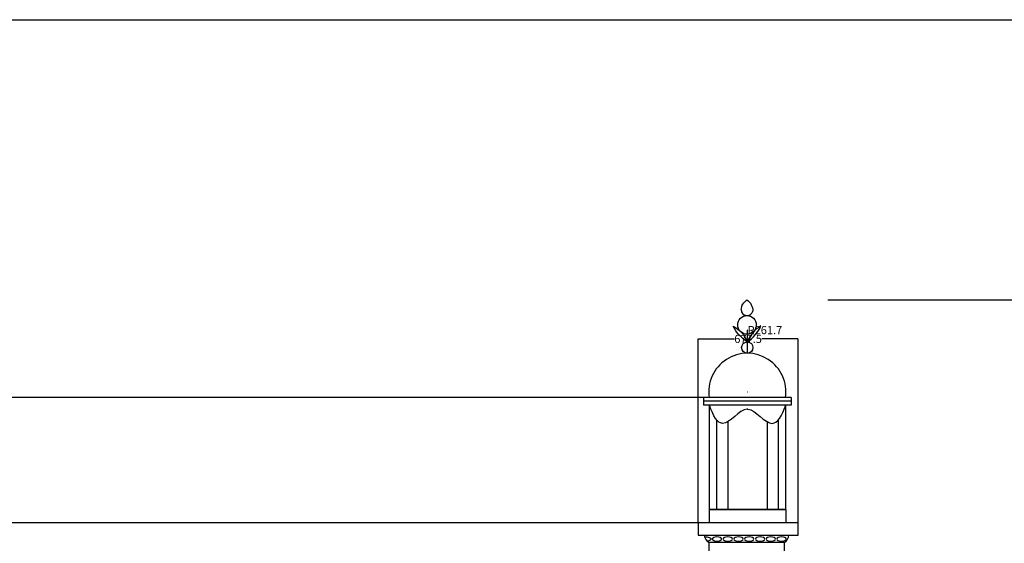
# Model space of a CAD drawing. Units: millimetres. Extents: x 8570 to 49085, y 3782 to 24863.
# Tile 11 of 15: x 28488 to 35169, y 17835 to 21387. Entities that reach past the tile are written whole.
import ezdxf

# ---------------------------------------------------------------- set-up
doc = ezdxf.new("R2010")
doc.units = ezdxf.units.MM
doc.header["$MEASUREMENT"] = 0
doc.header["$PDMODE"] = 3
doc.layers.add('A-ANNO-DIMS', color=2, linetype='Continuous', lineweight=18)
doc.layers.add('A-ELEV-MNRT', color=7, linetype='Continuous', lineweight=30)
doc.styles.get("Standard").update_dxf_attribs({"font": 'arial.ttf'})
doc.dimstyles.get("Standard").update_dxf_attribs({"dimtxt": 55, "dimasz": 0.18, "dimexe": 0.18, "dimexo": 0.0625, "dimgap": 0.09, "dimtad": 0, "dimtih": 1, "dimtoh": 1, "dimdec": 0, "dimzin": 0, "dimdsep": 46, "dimtxsty": 'Standard', "dimcen": 0.09, "dimadec": 0, "dimazin": 0, "dimtfac": 1, "dimtdec": 0, "dimtofl": 0, "dimtmove": 0, "dimatfit": 3, "dimfxl": 1, "dimtolj": 1, "dimtzin": 0, "dimarcsym": 0})

# ---------------------------------------------------------------- blocks, each defined once
blk = doc.blocks.new('MINARET-ELEV')
for p, q in [((851, 12922), (257.5, 12922)), ((257.5, 12922), (257.5, 12872)), ((851, 12897), (257.5, 12897)), ((851, 12922), (851, 12872)), ((851, 12872), (257.5, 12872)), ((298, 12162), (298, 12872)), ((556.7, 12843), (552, 12843)), ((815.5, 12162), (815.5, 12872)), ((348, 12162), (348, 12766.4)), ((765.5, 12162), (765.5, 12770.9)), ((423, 12162), (423, 12760.1)), ((690.5, 12162), (690.5, 12757.3)), ((815.5, 12162), (298, 12162)), ((807, 11939), (295, 11939))]:
    blk.add_line(p, q)
blk.add_lwpolyline([(512, 13519.5, -0.216309), (551.3, 13585.8, -0.244698), (591, 13509.3, -0.244698)], format="xyb")
for points in [[(554, 13300, -0.140093), (458.9, 13405.9, -0.184272)], [(554, 13300, 0.140093), (646.7, 13408, 0.184272)]]:
    blk.add_lwpolyline(points, format="xyb", close=True)
for points in [[(815.5, 12072.5), (298, 12072.5), (298, 12162), (815.5, 12162)], [(898, 12072.5), (220.5, 12072.5), (220.5, 11989.2), (898, 11989.2)]]:
    blk.add_lwpolyline(points, close=True)
for points in [[(235, 7939), (235, 8939), (255, 8939), (255, 9939), (275, 9939), (275, 10939), (295, 10939), (295, 11939)], [(867, 7939), (867, 8939), (847, 8939), (847, 9939), (827, 9939), (827, 10939), (807, 10939), (807, 11939)]]:
    blk.add_lwpolyline(points)
for centre, radius in [((552, 13415.4), 63.1), ((554, 13261.5), 38.5)]:
    blk.add_circle(centre, radius)
for centre, radius, start, end in [((552, 13518.5), 40.1, 178.61203, 346.69346), ((554, 12961.3), 261.7, 351.36698, 188.63302), ((330.8, 12000.6), 71.3, 189.21146, 239.80255), ((759.2, 12000.8), 78.1, 307.68318, 351.42034)]:
    blk.add_arc(centre, radius, start, end)
at = {"extrusion": (0, 0, -1)}
for centre, start_param, end_param in [((275.2, 11962.4), -1.939365, 1.327018), ((348.2, 11962.4), -6.283185, 0), ((421.2, 11962.4), -6.283185, 0), ((494.2, 11962.4), -6.283185, 0), ((567.2, 11962.4), -6.283185, 0), ((640.2, 11962.4), -6.283185, 0), ((713.2, 11962.4), -6.283185, 0), ((786.2, 11962.4), -6.283185, 0)]:
    blk.add_ellipse(centre, major_axis=(31.8, 0), ratio=0.472441, start_param=start_param, end_param=end_param, dxfattribs=at)
for points in [[(554.4, 12843), (553.6, 12843), (500.8, 12843), (391.9, 12680.1), (321.9, 12795.7), (298, 12872)], [(554.4, 12843), (555.2, 12843), (607.9, 12843), (716.8, 12680.1), (786.9, 12795.7), (815.5, 12872)]]:
    blk.add_open_spline(points, degree=3, knots=[136.061972, 136.061972, 136.061972, 136.061972, 139.000899, 330.944902, 463.724089, 463.724089, 463.724089, 463.724089])
blk = doc.blocks.new('*D15')
at = {"layer": 'A-ANNO-DIMS', "color": 0, "lineweight": -2, "transparency": 16777216}
for p, q in [((33971.1, 19487.3), (36009.1, 19487.3)), ((36008.9, 19487.1), (36008.9, 12722.6)), ((36008.9, 5901.7), (36008.9, 12666.2)), ((33971.1, 5901.5), (36009.1, 5901.5))]:
    blk.add_line(p, q, dxfattribs=at)
at = {"layer": 'A-ANNO-DIMS', "color": 0, "transparency": 16777216}
for points in [[(36008.8, 19487.1), (36008.9, 19487.1), (36008.9, 19487.3)], [(36008.8, 5901.7), (36008.9, 5901.7), (36008.9, 5901.5)]]:
    blk.add_solid(points, dxfattribs=at)
at = {"layer": 'Defpoints', "color": 0, "transparency": 16777216}
for p in [(33971, 19487.3), (36008.9, 19487.3), (33971, 5901.5)]:
    blk.add_point(p, dxfattribs=at)
at = {"layer": 'A-ANNO-DIMS', "color": 0, "transparency": 16777216, "insert": (36008.9, 12694.4), "char_height": 55, "attachment_point": 5}
blk.add_mtext('\\A1;MINARET 13586 TYP.', dxfattribs=at)
blk = doc.blocks.new('*D54')
at = {"layer": 'A-ANNO-DIMS', "color": 0, "lineweight": -2, "transparency": 16777216}
for p, q in [((24765.7, 21387.4), (36055.2, 21387.4)), ((36055, 21387.2), (36055, 19513.3)), ((36055, 17583), (36055, 19456.9)), ((26017.6, 17582.8), (36055.2, 17582.8))]:
    blk.add_line(p, q, dxfattribs=at)
at = {"layer": 'A-ANNO-DIMS', "color": 0, "transparency": 16777216}
for points in [[(36055, 21387.2), (36055, 21387.2), (36055, 21387.4)], [(36055, 17583), (36055, 17583), (36055, 17582.8)]]:
    blk.add_solid(points, dxfattribs=at)
at = {"layer": 'Defpoints', "color": 0, "transparency": 16777216}
for p in [(24765.6, 21387.4), (36055, 21387.4), (26017.6, 17582.8)]:
    blk.add_point(p, dxfattribs=at)
at = {"layer": 'A-ANNO-DIMS', "color": 0, "transparency": 16777216, "insert": (36055, 19485.1), "char_height": 55, "attachment_point": 5}
blk.add_mtext('\\A1;3804.6', dxfattribs=at)
blk = doc.blocks.new('*D61')
at = {"layer": 'A-ANNO-DIMS', "color": 0, "lineweight": -2, "transparency": 16777216}
for p, q in [((33091.4, 17974), (8684.3, 17974)), ((8684.5, 17973.8), (8684.5, 15935.4)), ((8684.5, 13840.7), (8684.5, 15879.1)), ((33041.4, 13840.5), (8684.3, 13840.5))]:
    blk.add_line(p, q, dxfattribs=at)
at = {"layer": 'A-ANNO-DIMS', "color": 0, "transparency": 16777216}
for points in [[(8684.5, 17973.8), (8684.5, 17973.8), (8684.5, 17974)], [(8684.5, 13840.7), (8684.5, 13840.7), (8684.5, 13840.5)]]:
    blk.add_solid(points, dxfattribs=at)
at = {"layer": 'Defpoints', "color": 0, "transparency": 16777216}
for p in [(8684.5, 17974), (33091.5, 17974), (33041.5, 13840.5)]:
    blk.add_point(p, dxfattribs=at)
at = {"layer": 'A-ANNO-DIMS', "color": 0, "transparency": 16777216, "insert": (8684.5, 15907.2), "char_height": 55, "attachment_point": 5}
blk.add_mtext('\\A1;4133.5', dxfattribs=at)
blk = doc.blocks.new('*D62')
at = {"layer": 'A-ANNO-DIMS', "color": 0, "lineweight": -2, "transparency": 16777216}
for p, q in [((33128.4, 18823.5), (8684.3, 18823.5)), ((8684.5, 18823.3), (8684.5, 18426.9)), ((8684.5, 17974.2), (8684.5, 18370.6)), ((33091.4, 17974), (8684.3, 17974))]:
    blk.add_line(p, q, dxfattribs=at)
at = {"layer": 'A-ANNO-DIMS', "color": 0, "transparency": 16777216}
for points in [[(8684.5, 18823.3), (8684.5, 18823.3), (8684.5, 18823.5)], [(8684.5, 17974.2), (8684.5, 17974.2), (8684.5, 17974)]]:
    blk.add_solid(points, dxfattribs=at)
at = {"layer": 'Defpoints', "color": 0, "transparency": 16777216}
for p in [(8684.5, 18823.5), (33128.5, 18823.5), (33091.5, 17974)]:
    blk.add_point(p, dxfattribs=at)
at = {"layer": 'A-ANNO-DIMS', "color": 0, "transparency": 16777216, "insert": (8684.5, 18398.7), "char_height": 55, "attachment_point": 5}
blk.add_mtext('\\A1;849.5', dxfattribs=at)
blk = doc.blocks.new('*D65')
at = {"layer": 'A-ANNO-DIMS', "color": 0, "lineweight": -2, "transparency": 16777216}
for p, q in [((33091.5, 17974.1), (33091.5, 19222.2)), ((33091.7, 19222), (33337, 19222)), ((33768.8, 19222), (33523.5, 19222)), ((33769, 17974.1), (33769, 19222.2))]:
    blk.add_line(p, q, dxfattribs=at)
at = {"layer": 'A-ANNO-DIMS', "color": 0, "transparency": 16777216}
for points in [[(33091.7, 19222), (33091.7, 19222), (33091.5, 19222)], [(33768.8, 19222), (33768.8, 19222), (33769, 19222)]]:
    blk.add_solid(points, dxfattribs=at)
at = {"layer": 'Defpoints', "color": 0, "transparency": 16777216}
for p in [(33769, 19222), (33091.5, 17974), (33769, 17974)]:
    blk.add_point(p, dxfattribs=at)
at = {"layer": 'A-ANNO-DIMS', "color": 0, "transparency": 16777216, "insert": (33430.2, 19222), "char_height": 55, "attachment_point": 5}
blk.add_mtext('\\A1;677.5', dxfattribs=at)
blk = doc.blocks.new('*D94')
at = {"layer": 'A-ANNO-DIMS', "color": 0, "lineweight": -2, "transparency": 16777216}
for p, q in [((33425.2, 19281.5), (33425, 19281.5)), ((33425, 19281.5), (33425, 19124.7)), ((33424.9, 18862.8), (33425.1, 18862.8)), ((33425, 18862.7), (33425, 18862.9))]:
    blk.add_line(p, q, dxfattribs=at)
at = {"layer": 'A-ANNO-DIMS', "color": 0, "transparency": 16777216}
blk.add_solid([(33425, 19124.7), (33425, 19124.7), (33425, 19124.5)], dxfattribs=at)
at = {"layer": 'Defpoints', "color": 0, "transparency": 16777216}
for p in [(33425, 19124.5), (33425, 18862.8)]:
    blk.add_point(p, dxfattribs=at)
at = {"layer": 'A-ANNO-DIMS', "color": 0, "transparency": 16777216, "insert": (33544.4, 19281.5), "char_height": 55, "attachment_point": 5}
blk.add_mtext('\\A1;R261.7', dxfattribs=at)

msp = doc.modelspace()

# ---------------------------------------------------------------- block references
at = {"layer": 'A-ELEV-MNRT'}
msp.add_blockref('MINARET-ELEV', (32871, 5901.5), dxfattribs=at)

# ---------------------------------------------------------------- dimensions: what is measured, and where the dimension line sits
at = {"layer": 'A-ANNO-DIMS'}
for base, p1, p2, picture, middle in [((36055, 21387.41), (26017.56, 17582.82), (24765.63, 21387.41), '*D54', (36055, 19485.11)), ((8684.5, 18823.5), (33091.5, 17974), (33128.5, 18823.5), '*D62', (8684.5, 18398.75)), ((8684.5, 17974), (33041.5, 13840.5), (33091.5, 17974), '*D61', (8684.5, 15907.25))]:
    dim = msp.add_linear_dim(base=base, p1=p1, p2=p2, angle=90, dimstyle='Standard', override={"dimdec": 1, "dimlfac": 1, "dimrnd": 0, "dimzin": 0, "dimdsep": 46, "dimlunit": 2}, dxfattribs=at)
    dim.commit()
    dim.dimension.update_dxf_attribs({"geometry": picture, "text_midpoint": middle})
dim = msp.add_linear_dim(base=(36008.87, 19487.32), p1=(33971, 5901.5), p2=(33971, 19487.32), angle=90, text='MINARET <> TYP.', dimstyle='Standard', override={"dimdec": 0, "dimlfac": 1, "dimrnd": 0, "dimzin": 0, "dimdsep": 46, "dimlunit": 2}, dxfattribs=at)
dim.commit()
dim.dimension.update_dxf_attribs({"geometry": '*D15', "text_midpoint": (36008.87, 12694.41)})
dim = msp.add_radius_dim(center=(33425, 18862.78), mpoint=(33425, 19124.5), dimstyle='Standard', override={"dimdec": 1, "dimlfac": 1, "dimrnd": 0, "dimzin": 0, "dimdsep": 46, "dimlunit": 2}, dxfattribs=at)
dim.commit()
dim.dimension.update_dxf_attribs({"geometry": '*D94', "text_midpoint": (33544.39, 19281.53), "dimtype": 164})
dim = msp.add_linear_dim(base=(33769, 19222), p1=(33091.5, 17974), p2=(33769, 17974), dimstyle='Standard', override={"dimdec": 1, "dimlfac": 1, "dimrnd": 0, "dimzin": 0, "dimdsep": 46, "dimlunit": 2}, dxfattribs=at)
dim.commit()
dim.dimension.update_dxf_attribs({"geometry": '*D65', "text_midpoint": (33430.25, 19222)})

doc.saveas('drawing.dxf')
